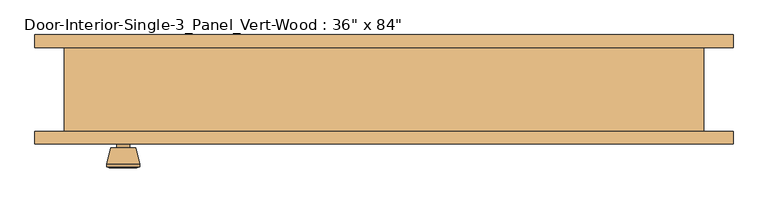
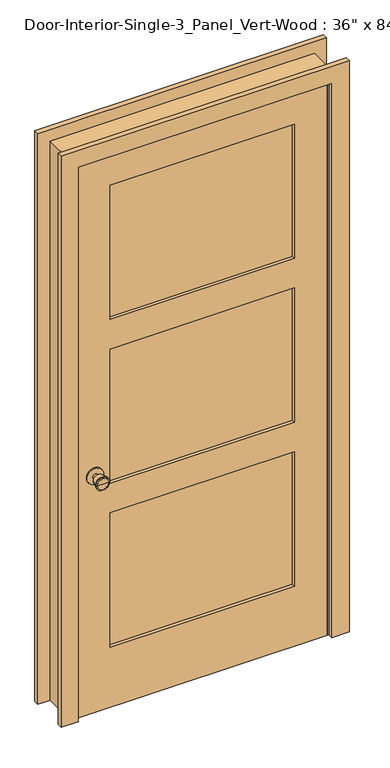
"""IFC4 building model written with IfcOpenShell, lengths in millimetres: door geometry."""

from ifc_helpers import new_model, si_unit, point, frame, frame_2d, origin, place, context, project, spatial, polyline, circle_curve, trimmed, segment, composite_curve, outline, extrude, faceted_brep, source, transform, mapped, element, save
from ifc_brep_helpers import plane_surface, cylinder_surface, revolved_surface, advanced_brep


def door_b31adefa(model_context):
    return source(origin(), model_context, "Body", "SolidModel", [
        advanced_brep(
        [(-393.7, -19.4, 914.4), (-403.7, -19.4, 914.4), (-383.7, -19.4, 914.4), (-373.2241324, 29.6, 914.4), (-414.1758676, 29.6, 914.4), (-393.7, 29.6, 914.4), (-368.7, 27.7721319, 914.4), (-418.7, 27.7721319, 914.4), (-368.7, 24.3084537, 914.4), (-418.7, 24.3084537, 914.4), (-375.063764, -0.4, 914.4), (-412.336236, -0.4, 914.4), (-383.7, -0.4, 914.4), (-403.7, -0.4, 914.4)],
        [
            (0, 1),
            (1, 2, circle_curve(frame((-393.7, -19.4, 914.4), z_axis=(0.0, -1.0, 0.0), x_axis=(-1.0, 0.0, 0.0)), 10.0)),
            (2, 0),
            (2, 1, circle_curve(frame((-393.7, -19.4, 914.4), z_axis=(0.0, -1.0, 0.0), x_axis=(-1.0, 0.0, 0.0)), 10.0)),
            (3, 4, circle_curve(frame((-393.7, 29.6, 914.4), z_axis=(0.0, 1.0, 0.0), x_axis=(-1.0, 0.0, 0.0)), 20.4758676)),
            (4, 5),
            (5, 3),
            (4, 3, circle_curve(frame((-393.7, 29.6, 914.4), z_axis=(0.0, 1.0, 0.0), x_axis=(-1.0, 0.0, 0.0)), 20.4758676)),
            (6, 7, circle_curve(frame((-393.7, 27.7721319, 914.4), z_axis=(0.0, 1.0, 0.0), x_axis=(-1.0, 0.0, 0.0)), 25.0)),
            (7, 4),
            (3, 6),
            (7, 6, circle_curve(frame((-393.7, 27.7721319, 914.4), z_axis=(0.0, 1.0, 0.0), x_axis=(-1.0, 0.0, 0.0)), 25.0)),
            (8, 9, circle_curve(frame((-393.7, 24.3084537, 914.4), z_axis=(0.0, 1.0, 0.0), x_axis=(-1.0, 0.0, 0.0)), 25.0)),
            (9, 7),
            (6, 8),
            (9, 8, circle_curve(frame((-393.7, 24.3084537, 914.4), z_axis=(0.0, 1.0, 0.0), x_axis=(-1.0, 0.0, 0.0)), 25.0)),
            (10, 11, circle_curve(frame((-393.7, -0.4, 914.4), z_axis=(0.0, 1.0, 0.0), x_axis=(-1.0, 0.0, 0.0)), 18.636236)),
            (11, 9),
            (8, 10),
            (11, 10, circle_curve(frame((-393.7, -0.4, 914.4), z_axis=(0.0, 1.0, 0.0), x_axis=(-1.0, 0.0, 0.0)), 18.636236)),
            (12, 13, circle_curve(frame((-393.7, -0.4, 914.4), z_axis=(0.0, 1.0, 0.0), x_axis=(-1.0, 0.0, 0.0)), 10.0)),
            (13, 11),
            (10, 12),
            (13, 12, circle_curve(frame((-393.7, -0.4, 914.4), z_axis=(0.0, 1.0, 0.0), x_axis=(-1.0, 0.0, 0.0)), 10.0)),
            (1, 13),
            (12, 2),
        ],
        [
            plane_surface(frame((-393.7, -19.4, 914.4), z_axis=(0.0, -1.0, 0.0), x_axis=(-1.0, 0.0, 0.0))),
            plane_surface(frame((-393.7, 29.6, 914.4), z_axis=(0.0, 1.0, 0.0), x_axis=(-1.0, 0.0, 0.0))),
            revolved_surface(polyline([(-414.1758676, 29.6, 914.4), (-418.7, 27.7721319, 914.4)]), (-393.7, -19.4, 914.4), (0.0, -1.0, 0.0)),
            cylinder_surface(frame((-393.7, -19.4, 914.4), z_axis=(0.0, -1.0, 0.0), x_axis=(-1.0, 0.0, 0.0)), 25.0),
            revolved_surface(polyline([(-418.7, 24.3084537, 914.4), (-412.336236, -0.4, 914.4)]), (-393.7, -19.4, 914.4), (0.0, -1.0, 0.0)),
            plane_surface(frame((-393.7, -0.4, 914.4), z_axis=(0.0, -1.0, 0.0), x_axis=(-1.0, 0.0, 0.0))),
            cylinder_surface(frame((-393.7, -19.4, 914.4), z_axis=(0.0, -1.0, 0.0), x_axis=(-1.0, 0.0, 0.0)), 10.0),
        ],
        [
            (0, [[1, 2, 3]]),
            (0, [[-3, 4, -1]]),
            (1, [[5, 6, 7]]),
            (1, [[8, -7, -6]]),
            (2, [[9, 10, -5, 11]]),
            (2, [[12, -11, -8, -10]]),
            (3, [[13, 14, -9, 15]]),
            (3, [[16, -15, -12, -14]]),
            (4, [[17, 18, -13, 19]]),
            (4, [[20, -19, -16, -18]]),
            (5, [[21, 22, -17, 23]]),
            (5, [[24, -23, -20, -22]]),
            (6, [[-2, 25, -21, 26]]),
            (6, [[-4, -26, -24, -25]]),
        ],
    ),
        extrude(outline(composite_curve([segment(trimmed(circle_curve(frame_2d((914.4, -393.7)), 30.0), [point((914.4, -423.7))], [point((914.4, -363.7))], False, "CARTESIAN"), True, "CONTINUOUS"), segment(trimmed(circle_curve(frame_2d((914.4, -393.7)), 30.0), [point((914.4, -363.7))], [point((914.4, -423.7))], False, "CARTESIAN"), True, "CONTINUOUS")], self_intersect=False)), frame((0.0, -25.4, 0.0), z_axis=(0.0, 1.0, 0.0), x_axis=(0.0, 0.0, 1.0)), (0.0, 0.0, 1.0), 6.0),
        advanced_brep(
        [(-393.7, -66.325, 914.4), (-383.7, -66.325, 914.4), (-403.7, -66.325, 914.4), (-373.2241324, -115.325, 914.4), (-393.7, -115.325, 914.4), (-414.1758676, -115.325, 914.4), (-368.7, -113.4971319, 914.4), (-418.7, -113.4971319, 914.4), (-368.7, -110.0334537, 914.4), (-418.7, -110.0334537, 914.4), (-375.063764, -85.325, 914.4), (-412.336236, -85.325, 914.4), (-383.7, -85.325, 914.4), (-403.7, -85.325, 914.4)],
        [
            (0, 1),
            (1, 2, circle_curve(frame((-393.7, -66.325, 914.4), z_axis=(0.0, 1.0, 0.0), x_axis=(-1.0, 0.0, 0.0)), 10.0)),
            (2, 0),
            (2, 1, circle_curve(frame((-393.7, -66.325, 914.4), z_axis=(0.0, 1.0, 0.0), x_axis=(-1.0, 0.0, 0.0)), 10.0)),
            (3, 4),
            (4, 5),
            (5, 3, circle_curve(frame((-393.7, -115.325, 914.4), z_axis=(0.0, -1.0, 0.0), x_axis=(-1.0, 0.0, 0.0)), 20.4758676)),
            (3, 5, circle_curve(frame((-393.7, -115.325, 914.4), z_axis=(0.0, -1.0, 0.0), x_axis=(-1.0, 0.0, 0.0)), 20.4758676)),
            (6, 3),
            (5, 7),
            (7, 6, circle_curve(frame((-393.7, -113.4971319, 914.4), z_axis=(0.0, -1.0, 0.0), x_axis=(-1.0, 0.0, 0.0)), 25.0)),
            (6, 7, circle_curve(frame((-393.7, -113.4971319, 914.4), z_axis=(0.0, -1.0, 0.0), x_axis=(-1.0, 0.0, 0.0)), 25.0)),
            (8, 6),
            (7, 9),
            (9, 8, circle_curve(frame((-393.7, -110.0334537, 914.4), z_axis=(0.0, -1.0, 0.0), x_axis=(-1.0, 0.0, 0.0)), 25.0)),
            (8, 9, circle_curve(frame((-393.7, -110.0334537, 914.4), z_axis=(0.0, -1.0, 0.0), x_axis=(-1.0, 0.0, 0.0)), 25.0)),
            (10, 8),
            (9, 11),
            (11, 10, circle_curve(frame((-393.7, -85.325, 914.4), z_axis=(0.0, -1.0, 0.0), x_axis=(-1.0, 0.0, 0.0)), 18.636236)),
            (10, 11, circle_curve(frame((-393.7, -85.325, 914.4), z_axis=(0.0, -1.0, 0.0), x_axis=(-1.0, 0.0, 0.0)), 18.636236)),
            (12, 10),
            (11, 13),
            (13, 12, circle_curve(frame((-393.7, -85.325, 914.4), z_axis=(0.0, -1.0, 0.0), x_axis=(-1.0, 0.0, 0.0)), 10.0)),
            (12, 13, circle_curve(frame((-393.7, -85.325, 914.4), z_axis=(0.0, -1.0, 0.0), x_axis=(-1.0, 0.0, 0.0)), 10.0)),
            (1, 12),
            (13, 2),
        ],
        [
            plane_surface(frame((-393.7, -66.325, 914.4), z_axis=(0.0, 1.0, 0.0), x_axis=(-1.0, 0.0, 0.0))),
            plane_surface(frame((-393.7, -115.325, 914.4), z_axis=(0.0, -1.0, 0.0), x_axis=(-1.0, 0.0, 0.0))),
            revolved_surface(polyline([(-414.1758676, -115.325, 914.4), (-418.7, -113.4971319, 914.4)]), (-393.7, -66.325, 914.4), (0.0, 1.0, 0.0)),
            cylinder_surface(frame((-393.7, -66.325, 914.4), z_axis=(0.0, 1.0, 0.0), x_axis=(-1.0, 0.0, 0.0)), 25.0),
            revolved_surface(polyline([(-418.7, -110.0334537, 914.4), (-412.336236, -85.325, 914.4)]), (-393.7, -66.325, 914.4), (0.0, 1.0, 0.0)),
            plane_surface(frame((-393.7, -85.325, 914.4), z_axis=(0.0, 1.0, 0.0), x_axis=(-1.0, 0.0, 0.0))),
            cylinder_surface(frame((-393.7, -66.325, 914.4), z_axis=(0.0, 1.0, 0.0), x_axis=(-1.0, 0.0, 0.0)), 10.0),
        ],
        [
            (0, [[1, 2, 3]]),
            (0, [[-3, 4, -1]]),
            (1, [[5, 6, 7]]),
            (1, [[-6, -5, 8]]),
            (2, [[9, -7, 10, 11]]),
            (2, [[-10, -8, -9, 12]]),
            (3, [[13, -11, 14, 15]]),
            (3, [[-14, -12, -13, 16]]),
            (4, [[17, -15, 18, 19]]),
            (4, [[-18, -16, -17, 20]]),
            (5, [[21, -19, 22, 23]]),
            (5, [[-22, -20, -21, 24]]),
            (6, [[25, -23, 26, -2]]),
            (6, [[-26, -24, -25, -4]]),
        ],
    ),
        extrude(outline(composite_curve([segment(trimmed(circle_curve(frame_2d((914.4, -393.7)), 30.0), [point((914.4, -423.7))], [point((914.4, -363.7))], False, "CARTESIAN"), True, "CONTINUOUS"), segment(trimmed(circle_curve(frame_2d((914.4, -393.7)), 30.0), [point((914.4, -363.7))], [point((914.4, -423.7))], False, "CARTESIAN"), True, "CONTINUOUS")], self_intersect=False)), frame((0.0, -66.325, 0.0), z_axis=(0.0, 1.0, 0.0), x_axis=(0.0, 0.0, 1.0)), (0.0, 0.0, 1.0), 6.0),
        faceted_brep([(482.6, -60.325, 0.0), (457.2, -60.325, 0.0), (457.2, -25.4, 0.0), (444.5, -25.4, 0.0), (444.5, 9.525, 0.0), (457.2, 9.525, 0.0), (457.2, 66.675, 0.0), (482.6, 66.675, 0.0), (482.6, 66.675, 2159.0), (482.6, -60.325, 2159.0), (457.2, 66.675, 2133.6), (-457.2, 66.675, 2133.6), (-457.2, 66.675, 0.0), (-482.6, 66.675, 0.0), (-482.6, 66.675, 2159.0), (457.2, 9.525, 2133.6), (444.5, 9.525, 2120.9), (-444.5, 9.525, 2120.9), (-444.5, 9.525, 0.0), (-457.2, 9.525, 0.0), (-457.2, 9.525, 2133.6), (444.5, -25.4, 2120.9), (457.2, -25.4, 2133.6), (-457.2, -25.4, 2133.6), (-457.2, -25.4, 0.0), (-444.5, -25.4, 0.0), (-444.5, -25.4, 2120.9), (457.2, -60.325, 2133.6), (-482.6, -60.325, 2159.0), (-482.6, -60.325, 0.0), (-457.2, -60.325, 0.0), (-457.2, -60.325, 2133.6)], [[[0, 1, 2, 3, 4, 5, 6, 7]], [[7, 8, 9, 0]], [[6, 10, 11, 12, 13, 14, 8, 7]], [[5, 15, 10, 6]], [[4, 16, 17, 18, 19, 20, 15, 5]], [[3, 21, 16, 4]], [[2, 22, 23, 24, 25, 26, 21, 3]], [[1, 27, 22, 2]], [[0, 9, 28, 29, 30, 31, 27, 1]], [[8, 14, 28, 9]], [[15, 20, 11, 10]], [[21, 26, 17, 16]], [[27, 31, 23, 22]], [[29, 13, 12, 19, 18, 25, 24, 30]], [[14, 13, 29, 28]], [[20, 19, 12, 11]], [[26, 25, 18, 17]], [[31, 30, 24, 23]]]),
        extrude(outline(polyline([(2133.6, -457.2), (0.0, -457.2), (0.0, 457.2), (2133.6, 457.2), (2133.6, -457.2)]), holes=[polyline([(2014.5375, -336.55), (2014.5375, 336.55), (1496.4833333, 336.55), (1496.4833333, -336.55), (2014.5375, -336.55)]), polyline([(749.8291667, -336.55), (749.8291667, 336.55), (231.775, 336.55), (231.775, -336.55), (749.8291667, -336.55)]), polyline([(1382.1833333, -336.55), (1382.1833333, 336.55), (864.1291667, 336.55), (864.1291667, -336.55), (1382.1833333, -336.55)])]), frame((0.0, -60.325, 0.0), z_axis=(0.0, 1.0, 0.0), x_axis=(0.0, 0.0, 1.0)), (0.0, 0.0, 1.0), 34.925),
        extrude(outline(polyline([(336.55, -37.0416667), (336.55, -48.6833333), (-336.55, -48.6833333), (-336.55, -37.0416667), (336.55, -37.0416667)])), frame((0.0, 0.0, 1496.4833333), z_axis=(0.0, 0.0, 1.0), x_axis=(1.0, 0.0, 0.0)), (0.0, 0.0, 1.0), 518.0541667),
        extrude(outline(polyline([(336.55, -37.0416667), (336.55, -48.6833333), (-336.55, -48.6833333), (-336.55, -37.0416667), (336.55, -37.0416667)])), frame((0.0, 0.0, 231.775), z_axis=(0.0, 0.0, 1.0), x_axis=(1.0, 0.0, 0.0)), (0.0, 0.0, 1.0), 518.0541667),
        extrude(outline(polyline([(336.55, -37.0416667), (336.55, -48.6833333), (-336.55, -48.6833333), (-336.55, -37.0416667), (336.55, -37.0416667)])), frame((0.0, 0.0, 864.1291667), z_axis=(0.0, 0.0, 1.0), x_axis=(1.0, 0.0, 0.0)), (0.0, 0.0, 1.0), 518.0541667),
        extrude(outline(polyline([(0.0, 527.05), (2203.45, 527.05), (2203.45, -527.05), (0.0, -527.05), (0.0, -463.55), (2139.95, -463.55), (2139.95, 463.55), (0.0, 463.55), (0.0, 527.05)])), frame((0.0, -79.375, 0.0), z_axis=(0.0, 1.0, 0.0), x_axis=(0.0, 0.0, 1.0)), (0.0, 0.0, 1.0), 19.05),
        extrude(outline(polyline([(0.0, 527.05), (2203.45, 527.05), (2203.45, -527.05), (0.0, -527.05), (0.0, -463.55), (2139.95, -463.55), (2139.95, 463.55), (0.0, 463.55), (0.0, 527.05)])), frame((0.0, 66.675, 0.0), z_axis=(0.0, 1.0, 0.0), x_axis=(0.0, 0.0, 1.0)), (0.0, 0.0, 1.0), 19.05),
    ])


if __name__ == "__main__":
    model = new_model("IFC4")
    model_context = context("Model", 3, world=origin())
    ifc_project = project(units=[si_unit("LENGTHUNIT", "METRE", prefix="MILLI")], contexts=[model_context])
    site = spatial("IfcSite", under=ifc_project)
    building = spatial("IfcBuilding", under=site)
    placement = place(None, origin())
    door_shape = door_b31adefa(model_context)
    element("IfcDoor", 1, ObjectType="Door-Interior-Single-3_Panel_Vert-Wood : 36\" x 84\"", at=placement, inside=building, context=model_context, shape_type="MappedRepresentation", body=[
        mapped(door_shape, transform((0.0, 0.0, 0.0), x_axis=(1.0, 0.0, 0.0), y_axis=(0.0, 1.0, 0.0), z_axis=(0.0, 0.0, 1.0))),
    ])
    save(model, "model.ifc")

# Revit data of these elements
# Type "Door-Interior-Single-3_Panel_Vert-Wood : 36\" x 84\""
#   Type Mark = "9"
#   Assembly Code = "C1020300"
#   Analytic Construction = "Wooden"
#   Top Rail = 0' - 4 11/16"
#   Thickness = 0' - 1 3/8"
#   Thermal Resistance (R) = 2.5876 (h·ft²·°F)/BTU
#   Swing Angle [instance default] = 90.00°
#   Stiles = 0' - 4 3/4"
#   Rough Width = 3' - 2"
#   Rough Height = 7' - 1"
#   Intermediate Rail = 0' - 4 1/2"
#   Height = 7' - 0"
#   Width = 3' - 0"
#   Heat Transfer Coefficient (U) = 0.3865 BTU/(h·ft²·°F)
#   Bottom Rail = 0' - 9 1/8"
#   Trim Material = Cherry
#   Panel Material = Cherry
#   Frame Material = Cherry
#   Door Handle Material = Aluminum
#   Visual Light Transmittance = 0
#   Solar Heat Gain Coefficient = 0
#   Wall Closure = (empty or 0)
#   Function = (empty or 0)
# Element 1 (IfcDoor, "Door-Interior-Single-3_Panel_Vert-Wood : 36\" x 84\"")
#   Materials on its faces: "Cherry", "Aluminum"
# Materials
#   "Cherry": class "Wood", colour RGB 226 177 128, transparency 0, Description = "Prunus Serotina", Cost = 0
#   "Aluminum": class "Metal", colour RGB 247 247 247, transparency 0, Description = "Aluminum 6061", Cost = 0
